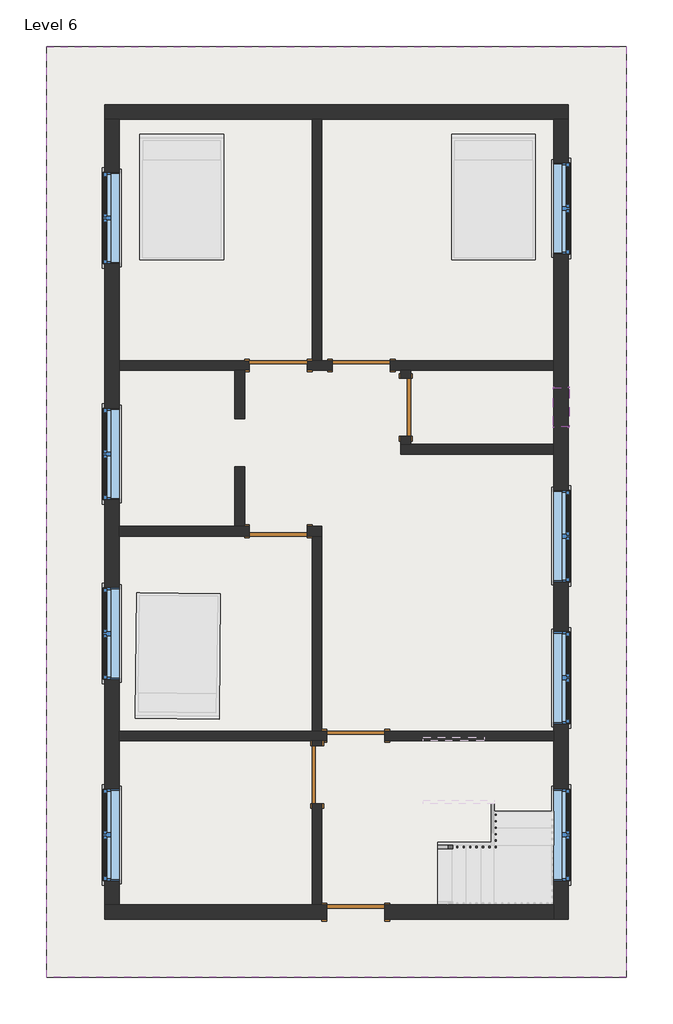
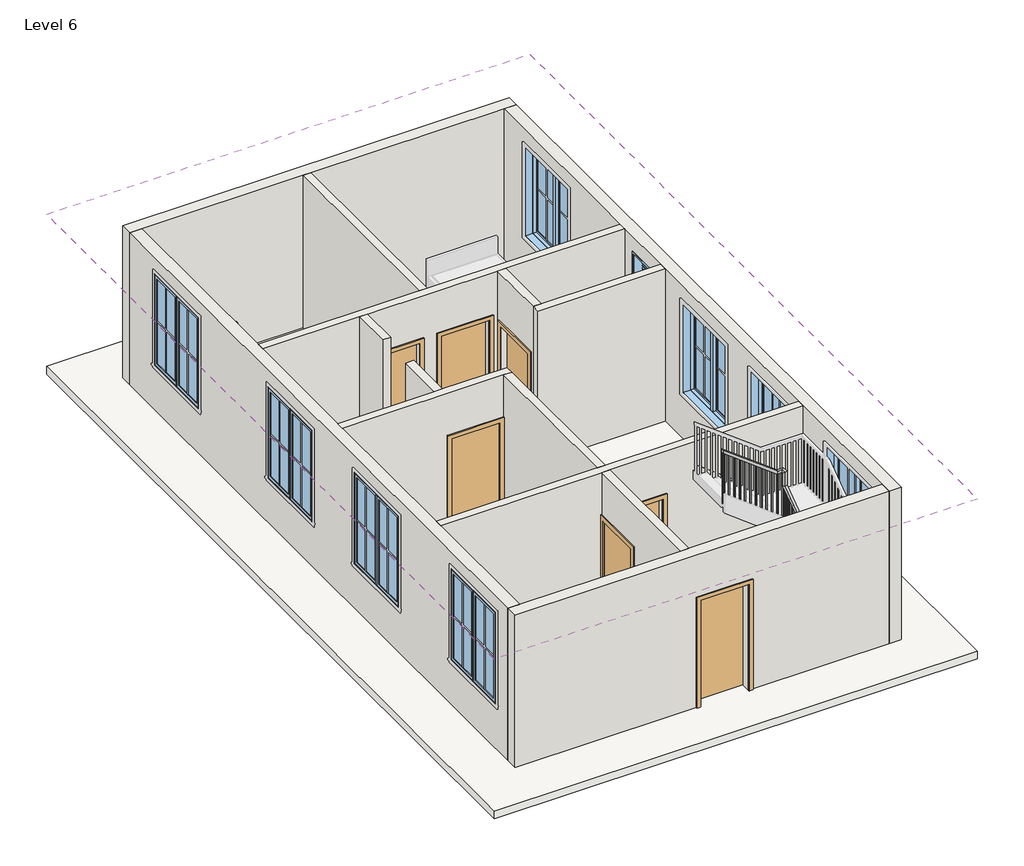
# One storey, part 1 of 2: 14 walls, 9 windows, 7 doors, 2 roofs, 1 railing.
"""IFC4 building model written with IfcOpenShell, lengths in millimetres."""

from ifc_helpers import new_model, si_unit, frame, origin, place, context, project, spatial, polyline, outline, extrude, faceted_brep, transform, mapped, element, save
from components import door_2b0b55a0, door_686f89d2, door_16372e1c, door_a90ba1ad, window_9ac97e1a, window_f2d8fef0

model = new_model("IFC4")

# Units and contexts
model_context = context("Model", 3, world=origin())
ifc_project = project(units=[si_unit("LENGTHUNIT", "METRE", prefix="MILLI")], contexts=[model_context])

# Site, building, storey
site = spatial("IfcSite", under=ifc_project)
building = spatial("IfcBuilding", under=site)
storey = spatial("IfcBuildingStorey", under=building, Name="Level 6", Elevation=12801.6)

# Doors
placement = place(None, origin())
door_shape = door_2b0b55a0(model_context)
element("IfcDoor", 1, ObjectType="Single-Flush : 36\" x 80\"", at=placement, inside=storey, context=model_context, shape_type="MappedRepresentation", body=[
    mapped(door_shape, transform((-163.235885, 1707.4649429, 12801.6), x_axis=(0.0, 1.0, 0.0), y_axis=(-1.0, 0.0, 0.0), z_axis=(0.0, 0.0, 1.0))),
])
door_2_shape = door_686f89d2(model_context)
element("IfcDoor", 2, ObjectType="Single-Flush : 36\" x 84\"", at=placement, inside=storey, context=model_context, shape_type="MappedRepresentation", body=[
    mapped(door_2_shape, transform((-861.735885, 2367.8649429, 12801.6), x_axis=(-1.0, 0.0, 0.0), y_axis=(0.0, -1.0, 0.0), z_axis=(0.0, 0.0, 1.0))),
])
element("IfcDoor", 3, ObjectType="Single-Flush : 36\" x 84\"", at=placement, inside=storey, context=model_context, shape_type="MappedRepresentation", body=[
    mapped(door_2_shape, transform((-2169.835885, -248.3350571, 12801.6), x_axis=(1.0, 0.0, 0.0), y_axis=(0.0, 1.0, 0.0), z_axis=(0.0, 0.0, 1.0))),
])
element("IfcDoor", 4, ObjectType="Single-Flush : 36\" x 84\"", at=placement, inside=storey, context=model_context, shape_type="MappedRepresentation", body=[
    mapped(door_2_shape, transform((-950.635885, -3474.1350571, 12801.6), x_axis=(-1.0, 0.0, 0.0), y_axis=(0.0, -1.0, 0.0), z_axis=(0.0, 0.0, 1.0))),
])
door_3_shape = door_16372e1c(model_context)
element("IfcDoor", 5, ObjectType="Single-Flush : 36\" x 84\"", at=placement, inside=storey, context=model_context, shape_type="MappedRepresentation", body=[
    mapped(door_3_shape, transform((-2169.835885, 2367.8649429, 12801.6), x_axis=(1.0, 0.0, 0.0), y_axis=(0.0, 1.0, 0.0), z_axis=(0.0, 0.0, 1.0))),
])
element("IfcDoor", 6, ObjectType="Single-Flush : 36\" x 84\"", at=placement, inside=storey, context=model_context, shape_type="MappedRepresentation", body=[
    mapped(door_3_shape, transform((-1560.235885, -4083.7350571, 12801.6), x_axis=(0.0, 1.0, 0.0), y_axis=(-1.0, 0.0, 0.0), z_axis=(0.0, 0.0, 1.0))),
])
door_4_shape = door_a90ba1ad(model_context)
element("IfcDoor", 7, ObjectType="Single-Flush : 36\" x 84\"", at=placement, inside=storey, context=model_context, shape_type="MappedRepresentation", body=[
    mapped(door_4_shape, transform((-950.635885, -6255.4350571, 12801.6), x_axis=(-1.0, 0.0, 0.0), y_axis=(0.0, -1.0, 0.0), z_axis=(0.0, 0.0, 1.0))),
])

# Railing
element("IfcRailing", 8, ObjectType="Handrail - Rectangular", at=placement, inside=storey, context=model_context, shape_type="SolidModel", body=[
    faceted_brep([(344.764115, -5201.3350571, 13885.3333333), (344.764115, -5201.3350571, 13821.4686436), (344.764115, -5252.1350571, 13821.4686436), (344.764115, -5252.1350571, 13885.3333333), (1157.564115, -5201.3350571, 14504.6095238), (1208.364115, -5201.3350571, 14479.449596), (1208.364115, -5252.1350571, 14479.449596), (1157.564115, -5252.1350571, 14504.6095238), (1157.564115, -5201.3350571, 14786.4285714), (1208.364115, -5201.3350571, 14735.6285714), (1208.364115, -5252.1350571, 14735.6285714), (1157.564115, -5252.1350571, 14786.4285714), (1233.764115, -5201.3350571, 14786.4285714), (1233.764115, -5201.3350571, 14735.6285714), (1284.564115, -5252.1350571, 14735.6285714), (1284.564115, -5252.1350571, 14786.4285714), (1233.764115, -5125.1350571, 14786.4285714), (1233.764115, -5108.8554323, 14735.6285714), (1284.564115, -5108.8554323, 14735.6285714), (1284.564115, -5125.1350571, 14786.4285714), (1233.764115, -4566.3350571, 15185.5714286), (1233.764115, -4515.5350571, 15159.4288395), (1284.564115, -4515.5350571, 15159.4288395), (1284.564115, -4566.3350571, 15185.5714286), (1233.764115, -4566.3350571, 15467.0606061), (1233.764115, -4515.5350571, 15416.2606061), (1284.564115, -4515.5350571, 15416.2606061), (1284.564115, -4566.3350571, 15467.0606061), (1233.764115, -4490.1350571, 15467.0606061), (1233.764115, -4490.1350571, 15416.2606061), (1284.564115, -4439.3350571, 15416.2606061), (1284.564115, -4439.3350571, 15467.0606061), (1157.564115, -4490.1350571, 15467.0606061), (1140.4943334, -4490.1350571, 15416.2606061), (1140.4943334, -4439.3350571, 15416.2606061), (1157.564115, -4439.3350571, 15467.0606061), (116.164115, -4490.1350571, 16256.0), (116.164115, -4439.3350571, 16256.0), (116.164115, -4439.3350571, 16192.2683472), (116.164115, -4490.1350571, 16192.2683472)], [[[0, 1, 2, 3]], [[1, 0, 4, 5]], [[2, 1, 5, 6]], [[3, 2, 6, 7]], [[0, 3, 7, 4]], [[5, 4, 8, 9]], [[6, 5, 9, 10]], [[7, 6, 10, 11]], [[4, 7, 11, 8]], [[9, 8, 12, 13]], [[10, 9, 13, 14]], [[11, 10, 14, 15]], [[8, 11, 15, 12]], [[13, 12, 16, 17]], [[14, 13, 17, 18]], [[15, 14, 18, 19]], [[12, 15, 19, 16]], [[17, 16, 20, 21]], [[18, 17, 21, 22]], [[19, 18, 22, 23]], [[16, 19, 23, 20]], [[21, 20, 24, 25]], [[22, 21, 25, 26]], [[23, 22, 26, 27]], [[20, 23, 27, 24]], [[25, 24, 28, 29]], [[26, 25, 29, 30]], [[27, 26, 30, 31]], [[24, 27, 31, 28]], [[29, 28, 32, 33]], [[30, 29, 33, 34]], [[31, 30, 34, 35]], [[28, 31, 35, 32]], [[36, 37, 38, 39]], [[33, 32, 36, 39]], [[34, 33, 39, 38]], [[35, 34, 38, 37]], [[32, 35, 37, 36]]]),
    extrude(outline(polyline([(16180.2418321, 132.039115), (15172.2666667, 132.039115), (15172.2666667, 151.089115), (16165.8100139, 151.089115), (16180.2418321, 132.039115)])), frame((0.0, -4474.2600571, 0.0), z_axis=(0.0, 1.0, 0.0), x_axis=(0.0, 0.0, 1.0)), (0.0, 0.0, 1.0), 19.05),
    extrude(outline(polyline([(16103.2721351, 233.639115), (15172.2666667, 233.639115), (15172.2666667, 252.689115), (16088.8403169, 252.689115), (16103.2721351, 233.639115)])), frame((0.0, -4474.2600571, 0.0), z_axis=(0.0, 1.0, 0.0), x_axis=(0.0, 0.0, 1.0)), (0.0, 0.0, 1.0), 19.05),
    extrude(outline(polyline([(16026.3024382, 335.239115), (15172.2666667, 335.239115), (15172.2666667, 354.289115), (16011.87062, 354.289115), (16026.3024382, 335.239115)])), frame((0.0, -4474.2600571, 0.0), z_axis=(0.0, 1.0, 0.0), x_axis=(0.0, 0.0, 1.0)), (0.0, 0.0, 1.0), 19.05),
    extrude(outline(polyline([(15949.3327412, 436.839115), (15002.9333333, 436.839115), (15002.9333333, 455.889115), (15934.900923, 455.889115), (15949.3327412, 436.839115)])), frame((0.0, -4474.2600571, 0.0), z_axis=(0.0, 1.0, 0.0), x_axis=(0.0, 0.0, 1.0)), (0.0, 0.0, 1.0), 19.05),
    extrude(outline(polyline([(15872.3630442, 538.439115), (15002.9333333, 538.439115), (15002.9333333, 557.489115), (15857.931226, 557.489115), (15872.3630442, 538.439115)])), frame((0.0, -4474.2600571, 0.0), z_axis=(0.0, 1.0, 0.0), x_axis=(0.0, 0.0, 1.0)), (0.0, 0.0, 1.0), 19.05),
    extrude(outline(polyline([(15795.3933472, 640.039115), (14833.6, 640.039115), (14833.6, 659.089115), (15780.9615291, 659.089115), (15795.3933472, 640.039115)])), frame((0.0, -4474.2600571, 0.0), z_axis=(0.0, 1.0, 0.0), x_axis=(0.0, 0.0, 1.0)), (0.0, 0.0, 1.0), 19.05),
    extrude(outline(polyline([(15718.4236503, 741.639115), (14833.6, 741.639115), (14833.6, 760.689115), (15703.9918321, 760.689115), (15718.4236503, 741.639115)])), frame((0.0, -4474.2600571, 0.0), z_axis=(0.0, 1.0, 0.0), x_axis=(0.0, 0.0, 1.0)), (0.0, 0.0, 1.0), 19.05),
    extrude(outline(polyline([(15641.4539533, 843.239115), (14664.2666667, 843.239115), (14664.2666667, 862.289115), (15627.0221351, 862.289115), (15641.4539533, 843.239115)])), frame((0.0, -4474.2600571, 0.0), z_axis=(0.0, 1.0, 0.0), x_axis=(0.0, 0.0, 1.0)), (0.0, 0.0, 1.0), 19.05),
    extrude(outline(polyline([(15564.4842563, 944.839115), (14664.2666667, 944.839115), (14664.2666667, 963.889115), (15550.0524382, 963.889115), (15564.4842563, 944.839115)])), frame((0.0, -4474.2600571, 0.0), z_axis=(0.0, 1.0, 0.0), x_axis=(0.0, 0.0, 1.0)), (0.0, 0.0, 1.0), 19.05),
    extrude(outline(polyline([(15487.5145594, 1046.439115), (14494.9333333, 1046.439115), (14494.9333333, 1065.489115), (15473.0827412, 1065.489115), (15487.5145594, 1046.439115)])), frame((0.0, -4474.2600571, 0.0), z_axis=(0.0, 1.0, 0.0), x_axis=(0.0, 0.0, 1.0)), (0.0, 0.0, 1.0), 19.05),
    extrude(outline(polyline([(15410.5448624, 1148.039115), (14494.9333333, 1148.039115), (14494.9333333, 1167.089115), (15396.1130442, 1167.089115), (15410.5448624, 1148.039115)])), frame((0.0, -4474.2600571, 0.0), z_axis=(0.0, 1.0, 0.0), x_axis=(0.0, 0.0, 1.0)), (0.0, 0.0, 1.0), 19.05),
    extrude(outline(polyline([(1249.639115, -4525.0600571), (1249.639115, -4506.0100571), (1268.689115, -4506.0100571), (1268.689115, -4525.0600571), (1249.639115, -4525.0600571)])), frame((0.0, 0.0, 14156.2666667), z_axis=(0.0, 0.0, 1.0), x_axis=(1.0, 0.0, 0.0)), (0.0, 0.0, 1.0), 1259.9939394),
    extrude(outline(polyline([(-4607.6100571, 15093.6609823), (-4607.6100571, 14156.2666667), (-4626.6600571, 14156.2666667), (-4626.6600571, 15080.0538395), (-4607.6100571, 15093.6609823)])), frame((1249.639115, 0.0, 0.0), z_axis=(1.0, 0.0, 0.0), x_axis=(0.0, 1.0, 0.0)), (0.0, 0.0, 1.0), 19.05),
    extrude(outline(polyline([(-4709.2100571, 15021.0895538), (-4709.2100571, 13986.9333333), (-4728.2600571, 13986.9333333), (-4728.2600571, 15007.4824109), (-4709.2100571, 15021.0895538)])), frame((1249.639115, 0.0, 0.0), z_axis=(1.0, 0.0, 0.0), x_axis=(0.0, 1.0, 0.0)), (0.0, 0.0, 1.0), 19.05),
    extrude(outline(polyline([(-4810.8100571, 14948.5181252), (-4810.8100571, 13986.9333333), (-4829.8600571, 13986.9333333), (-4829.8600571, 14934.9109823), (-4810.8100571, 14948.5181252)])), frame((1249.639115, 0.0, 0.0), z_axis=(1.0, 0.0, 0.0), x_axis=(0.0, 1.0, 0.0)), (0.0, 0.0, 1.0), 19.05),
    extrude(outline(polyline([(-4912.4100571, 14875.9466966), (-4912.4100571, 13986.9333333), (-4931.4600571, 13986.9333333), (-4931.4600571, 14862.3395538), (-4912.4100571, 14875.9466966)])), frame((1249.639115, 0.0, 0.0), z_axis=(1.0, 0.0, 0.0), x_axis=(0.0, 1.0, 0.0)), (0.0, 0.0, 1.0), 19.05),
    extrude(outline(polyline([(-5014.0100571, 14803.3752681), (-5014.0100571, 13817.6), (-5033.0600571, 13817.6), (-5033.0600571, 14789.7681252), (-5014.0100571, 14803.3752681)])), frame((1249.639115, 0.0, 0.0), z_axis=(1.0, 0.0, 0.0), x_axis=(0.0, 1.0, 0.0)), (0.0, 0.0, 1.0), 19.05),
    extrude(outline(polyline([(-5115.6100571, 14730.8038395), (-5115.6100571, 13817.6), (-5134.6600571, 13817.6), (-5134.6600571, 14717.1966966), (-5115.6100571, 14730.8038395)])), frame((1249.639115, 0.0, 0.0), z_axis=(1.0, 0.0, 0.0), x_axis=(0.0, 1.0, 0.0)), (0.0, 0.0, 1.0), 19.05),
    extrude(outline(polyline([(14433.4876912, 1148.039115), (13478.9333333, 1148.039115), (13478.9333333, 1167.089115), (14448.0019769, 1167.089115), (14433.4876912, 1148.039115)])), frame((0.0, -5236.2600571, 0.0), z_axis=(0.0, 1.0, 0.0), x_axis=(0.0, 0.0, 1.0)), (0.0, 0.0, 1.0), 19.05),
    extrude(outline(polyline([(14356.0781674, 1046.439115), (13478.9333333, 1046.439115), (13478.9333333, 1065.489115), (14370.5924531, 1065.489115), (14356.0781674, 1046.439115)])), frame((0.0, -5236.2600571, 0.0), z_axis=(0.0, 1.0, 0.0), x_axis=(0.0, 0.0, 1.0)), (0.0, 0.0, 1.0), 19.05),
    extrude(outline(polyline([(14278.6686436, 944.839115), (13309.6, 944.839115), (13309.6, 963.889115), (14293.1829293, 963.889115), (14278.6686436, 944.839115)])), frame((0.0, -5236.2600571, 0.0), z_axis=(0.0, 1.0, 0.0), x_axis=(0.0, 0.0, 1.0)), (0.0, 0.0, 1.0), 19.05),
    extrude(outline(polyline([(14201.2591198, 843.239115), (13309.6, 843.239115), (13309.6, 862.289115), (14215.7734055, 862.289115), (14201.2591198, 843.239115)])), frame((0.0, -5236.2600571, 0.0), z_axis=(0.0, 1.0, 0.0), x_axis=(0.0, 0.0, 1.0)), (0.0, 0.0, 1.0), 19.05),
    extrude(outline(polyline([(14123.849596, 741.639115), (13140.2666667, 741.639115), (13140.2666667, 760.689115), (14138.3638817, 760.689115), (14123.849596, 741.639115)])), frame((0.0, -5236.2600571, 0.0), z_axis=(0.0, 1.0, 0.0), x_axis=(0.0, 0.0, 1.0)), (0.0, 0.0, 1.0), 19.05),
    extrude(outline(polyline([(14046.4400722, 640.039115), (13140.2666667, 640.039115), (13140.2666667, 659.089115), (14060.9543579, 659.089115), (14046.4400722, 640.039115)])), frame((0.0, -5236.2600571, 0.0), z_axis=(0.0, 1.0, 0.0), x_axis=(0.0, 0.0, 1.0)), (0.0, 0.0, 1.0), 19.05),
    extrude(outline(polyline([(13969.0305484, 538.439115), (12970.9333333, 538.439115), (12970.9333333, 557.489115), (13983.5448341, 557.489115), (13969.0305484, 538.439115)])), frame((0.0, -5236.2600571, 0.0), z_axis=(0.0, 1.0, 0.0), x_axis=(0.0, 0.0, 1.0)), (0.0, 0.0, 1.0), 19.05),
    extrude(outline(polyline([(13891.6210246, 436.839115), (12970.9333333, 436.839115), (12970.9333333, 455.889115), (13906.1353103, 455.889115), (13891.6210246, 436.839115)])), frame((0.0, -5236.2600571, 0.0), z_axis=(0.0, 1.0, 0.0), x_axis=(0.0, 0.0, 1.0)), (0.0, 0.0, 1.0), 19.05),
    extrude(outline(polyline([(1249.639115, -4474.2600571), (1249.639115, -4455.2100571), (1268.689115, -4455.2100571), (1268.689115, -4474.2600571), (1249.639115, -4474.2600571)])), frame((0.0, 0.0, 14325.6), z_axis=(0.0, 0.0, 1.0), x_axis=(1.0, 0.0, 0.0)), (0.0, 0.0, 1.0), 1090.6606061),
    extrude(outline(polyline([(1249.639115, -5217.2100571), (1268.689115, -5217.2100571), (1268.689115, -5236.2600571), (1249.639115, -5236.2600571), (1249.639115, -5217.2100571)])), frame((0.0, 0.0, 13648.2666667), z_axis=(0.0, 0.0, 1.0), x_axis=(1.0, 0.0, 0.0)), (0.0, 0.0, 1.0), 1087.3619048),
    extrude(outline(polyline([(16192.2683472, 116.164115), (15172.2666667, 116.164115), (15172.2666667, 135.214115), (16177.8365291, 135.214115), (16192.2683472, 116.164115)])), frame((0.0, -4474.2600571, 0.0), z_axis=(0.0, 1.0, 0.0), x_axis=(0.0, 0.0, 1.0)), (0.0, 0.0, 1.0), 19.05),
    extrude(outline(polyline([(13821.4686436, 344.764115), (12970.9333333, 344.764115), (12970.9333333, 363.814115), (13835.9829293, 363.814115), (13821.4686436, 344.764115)])), frame((0.0, -5236.2600571, 0.0), z_axis=(0.0, 1.0, 0.0), x_axis=(0.0, 0.0, 1.0)), (0.0, 0.0, 1.0), 19.05),
])

# Roofs
element("IfcRoof", 9, ObjectType="ROOF 6\"", at=placement, inside=storey, context=model_context, shape_type="SweptSolid", body=[
    extrude(outline(polyline([(-5827.435885, 7397.0649429), (3316.564115, 7397.0649429), (3316.564115, -7284.1350571), (-5827.435885, -7284.1350571), (-5827.435885, 7397.0649429)])), frame((0.0, 0.0, 12649.2), z_axis=(0.0, 0.0, 1.0), x_axis=(1.0, 0.0, 0.0)), (0.0, 0.0, 1.0), 152.4),
])
element("IfcRoof", 10, ObjectType="ROOF 6\"", at=placement, inside=storey, context=model_context, shape_type="SweptSolid", body=[
    extrude(outline(polyline([(-5827.435885, 7397.0649429), (3316.564115, 7397.0649429), (3316.564115, -7284.1350571), (-5827.435885, -7284.1350571), (-5827.435885, 7397.0649429)])), frame((0.0, 0.0, 15849.6), z_axis=(0.0, 0.0, 1.0), x_axis=(1.0, 0.0, 0.0)), (0.0, 0.0, 1.0), 152.4),
])

# Walls
element("IfcWall", 11, ObjectType="WALL 6\"", at=placement, inside=storey, context=model_context, shape_type="SweptSolid", body=[
    extrude(outline(polyline([(-1636.435885, 2444.0649429), (-1636.435885, 6254.0649429), (-1484.035885, 6254.0649429), (-1484.035885, 2444.0649429), (-1636.435885, 2444.0649429)])), frame((0.0, 0.0, 12801.6), z_axis=(0.0, 0.0, 1.0), x_axis=(1.0, 0.0, 0.0)), (0.0, 0.0, 1.0), 3048.0),
])
element("IfcWall", 12, ObjectType="WALL 6\"", at=placement, inside=storey, context=model_context, shape_type="Brep", body=[
    faceted_brep([(-1318.935885, 2444.0649429, 12801.6), (-1484.035885, 2444.0649429, 12801.6), (-1636.435885, 2444.0649429, 12801.6), (-1712.635885, 2444.0649429, 12801.6), (-1712.635885, 2444.0649429, 14935.2), (-2627.035885, 2444.0649429, 14935.2), (-2627.035885, 2444.0649429, 12801.6), (-4684.435885, 2444.0649429, 12801.6), (-4684.435885, 2444.0649429, 15849.6), (-1636.435885, 2444.0649429, 15849.6), (-1484.035885, 2444.0649429, 15849.6), (2173.564115, 2444.0649429, 15849.6), (2173.564115, 2444.0649429, 12801.6), (-404.535885, 2444.0649429, 12801.6), (-404.535885, 2444.0649429, 14935.2), (-1318.935885, 2444.0649429, 14935.2), (-1712.635885, 2291.6649429, 14935.2), (-1712.635885, 2291.6649429, 12801.6), (-1318.935885, 2291.6649429, 12801.6), (-1318.935885, 2291.6649429, 14935.2), (-404.535885, 2291.6649429, 14935.2), (-404.535885, 2291.6649429, 12801.6), (-239.435885, 2291.6649429, 12801.6), (-87.035885, 2291.6649429, 12801.6), (2173.564115, 2291.6649429, 12801.6), (2173.564115, 2291.6649429, 15849.6), (-87.035885, 2291.6649429, 15849.6), (-239.435885, 2291.6649429, 15849.6), (-2703.235885, 2291.6649429, 15849.6), (-2855.635885, 2291.6649429, 15849.6), (-4684.435885, 2291.6649429, 15849.6), (-4684.435885, 2291.6649429, 12801.6), (-2855.635885, 2291.6649429, 12801.6), (-2703.235885, 2291.6649429, 12801.6), (-2627.035885, 2291.6649429, 12801.6), (-2627.035885, 2291.6649429, 14935.2)], [[[0, 1, 2, 3, 4, 5, 6, 7, 8, 9, 10, 11, 12, 13, 14, 15]], [[16, 17, 18, 19, 20, 21, 22, 23, 24, 25, 26, 27, 28, 29, 30, 31, 32, 33, 34, 35]], [[13, 12, 24, 23, 22, 21]], [[18, 17, 3, 2, 1, 0]], [[34, 33, 32, 31, 7, 6]], [[12, 11, 25, 24]], [[8, 7, 31, 30]], [[19, 18, 0, 15]], [[20, 19, 15, 14]], [[21, 20, 14, 13]], [[4, 3, 17, 16]], [[5, 4, 16, 35]], [[6, 5, 35, 34]], [[11, 10, 9, 8, 30, 29, 28, 27, 26, 25]]]),
])
element("IfcWall", 13, ObjectType="WALL 6\"", at=placement, inside=storey, context=model_context, shape_type="SweptSolid", body=[
    extrude(outline(polyline([(-2855.635885, 1529.6649429), (-2855.635885, 2291.6649429), (-2703.235885, 2291.6649429), (-2703.235885, 1529.6649429), (-2855.635885, 1529.6649429)])), frame((0.0, 0.0, 12801.6), z_axis=(0.0, 0.0, 1.0), x_axis=(1.0, 0.0, 0.0)), (0.0, 0.0, 1.0), 3048.0),
])
element("IfcWall", 14, ObjectType="WALL 6\"", at=placement, inside=storey, context=model_context, shape_type="Brep", body=[
    faceted_brep([(-1712.635885, -324.5350571, 14935.2), (-1712.635885, -324.5350571, 12801.6), (-1636.435885, -324.5350571, 12801.6), (-1484.035885, -324.5350571, 12801.6), (-1484.035885, -324.5350571, 15849.6), (-1636.435885, -324.5350571, 15849.6), (-4684.435885, -324.5350571, 15849.6), (-4684.435885, -324.5350571, 12801.6), (-2627.035885, -324.5350571, 12801.6), (-2627.035885, -324.5350571, 14935.2), (-1484.035885, -172.1350571, 12801.6), (-1712.635885, -172.1350571, 12801.6), (-1712.635885, -172.1350571, 14935.2), (-2627.035885, -172.1350571, 14935.2), (-2627.035885, -172.1350571, 12801.6), (-2703.235885, -172.1350571, 12801.6), (-2855.635885, -172.1350571, 12801.6), (-4684.435885, -172.1350571, 12801.6), (-4684.435885, -172.1350571, 15849.6), (-2855.635885, -172.1350571, 15849.6), (-2703.235885, -172.1350571, 15849.6), (-1484.035885, -172.1350571, 15849.6)], [[[0, 1, 2, 3, 4, 5, 6, 7, 8, 9]], [[10, 11, 12, 13, 14, 15, 16, 17, 18, 19, 20, 21]], [[8, 7, 17, 16, 15, 14]], [[3, 2, 1, 11, 10]], [[7, 6, 18, 17]], [[4, 3, 10, 21]], [[12, 11, 1, 0]], [[13, 12, 0, 9]], [[14, 13, 9, 8]], [[6, 5, 4, 21, 20, 19, 18]]]),
])
element("IfcWall", 15, ObjectType="WALL 6\"", at=placement, inside=storey, context=model_context, shape_type="SweptSolid", body=[
    extrude(outline(polyline([(-1636.435885, -3397.9350571), (-1636.435885, -324.5350571), (-1484.035885, -324.5350571), (-1484.035885, -3397.9350571), (-1636.435885, -3397.9350571)])), frame((0.0, 0.0, 12801.6), z_axis=(0.0, 0.0, 1.0), x_axis=(1.0, 0.0, 0.0)), (0.0, 0.0, 1.0), 3048.0),
])
element("IfcWall", 16, ObjectType="WALL 6\"", at=placement, inside=storey, context=model_context, shape_type="Brep", body=[
    faceted_brep([(-4684.435885, -3550.3350571, 12801.6), (-1636.435885, -3550.3350571, 12801.6), (-1484.035885, -3550.3350571, 12801.6), (-1407.835885, -3550.3350571, 12801.6), (-1407.835885, -3550.3350571, 14935.2), (-493.435885, -3550.3350571, 14935.2), (-493.435885, -3550.3350571, 12801.6), (2173.564115, -3550.3350571, 12801.6), (2173.564115, -3550.3350571, 15849.6), (-1484.035885, -3550.3350571, 15849.6), (-1636.435885, -3550.3350571, 15849.6), (-4684.435885, -3550.3350571, 15849.6), (-1407.835885, -3397.9350571, 14935.2), (-1407.835885, -3397.9350571, 12801.6), (-1484.035885, -3397.9350571, 12801.6), (-1636.435885, -3397.9350571, 12801.6), (-4684.435885, -3397.9350571, 12801.6), (-4684.435885, -3397.9350571, 15849.6), (-1636.435885, -3397.9350571, 15849.6), (-1484.035885, -3397.9350571, 15849.6), (2173.564115, -3397.9350571, 15849.6), (2173.564115, -3397.9350571, 12801.6), (-493.435885, -3397.9350571, 12801.6), (-493.435885, -3397.9350571, 14935.2)], [[[0, 1, 2, 3, 4, 5, 6, 7, 8, 9, 10, 11]], [[12, 13, 14, 15, 16, 17, 18, 19, 20, 21, 22, 23]], [[22, 21, 7, 6]], [[16, 15, 14, 13, 3, 2, 1, 0]], [[8, 7, 21, 20]], [[0, 11, 17, 16]], [[4, 3, 13, 12]], [[5, 4, 12, 23]], [[6, 5, 23, 22]], [[11, 10, 9, 8, 20, 19, 18, 17]]]),
])
element("IfcWall", 17, ObjectType="WALL 6\"", at=placement, inside=storey, context=model_context, shape_type="SweptSolid", body=[
    extrude(outline(polyline([(-3550.3350571, 12801.6), (-3626.5350571, 12801.6), (-3626.5350571, 14935.2), (-4540.9350571, 14935.2), (-4540.9350571, 12801.6), (-6141.1350571, 12801.6), (-6141.1350571, 15849.6), (-3550.3350571, 15849.6), (-3550.3350571, 12801.6)])), frame((-1636.435885, 0.0, 0.0), z_axis=(1.0, 0.0, 0.0), x_axis=(0.0, 1.0, 0.0)), (0.0, 0.0, 1.0), 152.4),
])
element("IfcWall", 18, ObjectType="WALL 6\"", at=placement, inside=storey, context=model_context, shape_type="Brep", body=[
    faceted_brep([(2173.564115, 1123.2649429, 12801.6), (-87.035885, 1123.2649429, 12801.6), (-239.435885, 1123.2649429, 12801.6), (-239.435885, 1123.2649429, 15849.6), (-87.035885, 1123.2649429, 15849.6), (2173.564115, 1123.2649429, 15849.6), (2173.564115, 970.8649429, 12801.6), (2173.564115, 970.8649429, 15849.6), (-239.435885, 970.8649429, 15849.6), (-239.435885, 970.8649429, 12801.6)], [[[0, 1, 2, 3, 4, 5]], [[6, 7, 8, 9]], [[2, 1, 0, 6, 9]], [[0, 5, 7, 6]], [[3, 2, 9, 8]], [[5, 4, 3, 8, 7]]]),
])
element("IfcWall", 19, ObjectType="WALL 6\"", at=placement, inside=storey, context=model_context, shape_type="SweptSolid", body=[
    extrude(outline(polyline([(2291.6649429, 12801.6), (2164.6649429, 12801.6), (2164.6649429, 14833.6), (1250.2649429, 14833.6), (1250.2649429, 12801.6), (1123.2649429, 12801.6), (1123.2649429, 15849.6), (2291.6649429, 15849.6), (2291.6649429, 12801.6)])), frame((-239.435885, 0.0, 0.0), z_axis=(1.0, 0.0, 0.0), x_axis=(0.0, 1.0, 0.0)), (0.0, 0.0, 1.0), 152.4),
])
element("IfcWall", 20, ObjectType="WALL 6\"", at=placement, inside=storey, context=model_context, shape_type="SweptSolid", body=[
    extrude(outline(polyline([(-2855.635885, -172.1350571), (-2855.635885, 767.6649429), (-2703.235885, 767.6649429), (-2703.235885, -172.1350571), (-2855.635885, -172.1350571)])), frame((0.0, 0.0, 12801.6), z_axis=(0.0, 0.0, 1.0), x_axis=(1.0, 0.0, 0.0)), (0.0, 0.0, 1.0), 3048.0),
])
element("IfcWall", 21, ObjectType="WALL 9\"", at=placement, inside=storey, context=model_context, shape_type="Brep", body=[
    faceted_brep([(-4913.035885, 6254.0649429, 12801.6), (-4684.435885, 6254.0649429, 12801.6), (-1636.435885, 6254.0649429, 12801.6), (-1484.035885, 6254.0649429, 12801.6), (2173.564115, 6254.0649429, 12801.6), (2402.164115, 6254.0649429, 12801.6), (2402.164115, 6254.0649429, 15849.6), (2173.564115, 6254.0649429, 15849.6), (-1484.035885, 6254.0649429, 15849.6), (-1636.435885, 6254.0649429, 15849.6), (-4684.435885, 6254.0649429, 15849.6), (-4913.035885, 6254.0649429, 15849.6), (-4913.035885, 6482.6649429, 12801.6), (-4913.035885, 6482.6649429, 15849.6), (2402.164115, 6482.6649429, 15849.6), (2402.164115, 6482.6649429, 12801.6)], [[[0, 1, 2, 3, 4, 5, 6, 7, 8, 9, 10, 11]], [[12, 13, 14, 15]], [[5, 4, 3, 2, 1, 0, 12, 15]], [[6, 5, 15, 14]], [[0, 11, 13, 12]], [[11, 10, 9, 8, 7, 6, 14, 13]]]),
])
element("IfcWall", 22, ObjectType="WALL 9\"", at=placement, inside=storey, context=model_context, shape_type="Brep", body=[
    faceted_brep([(2173.564115, 6254.0649429, 12801.6), (2173.564115, 2444.0649429, 12801.6), (2173.564115, 2291.6649429, 12801.6), (2173.564115, 1123.2649429, 12801.6), (2173.564115, 970.8649429, 12801.6), (2173.564115, -3397.9350571, 12801.6), (2173.564115, -3550.3350571, 12801.6), (2173.564115, -6141.1350571, 12801.6), (2173.564115, -6369.7350571, 12801.6), (2173.564115, -6369.7350571, 15849.6), (2173.564115, -6141.1350571, 15849.6), (2173.564115, -3550.3350571, 15849.6), (2173.564115, -3397.9350571, 15849.6), (2173.564115, 970.8649429, 15849.6), (2173.564115, 1123.2649429, 15849.6), (2173.564115, 2291.6649429, 15849.6), (2173.564115, 2444.0649429, 15849.6), (2173.564115, 6254.0649429, 15849.6), (2173.564115, -5760.1350571, 15544.8), (2173.564115, -5760.1350571, 13716.0), (2173.564115, -4312.3350571, 13716.0), (2173.564115, -4312.3350571, 15544.8), (2173.564115, -3283.6350571, 15544.8), (2173.564115, -3283.6350571, 13716.0), (2173.564115, -1835.8350571, 13716.0), (2173.564115, -1835.8350571, 15544.8), (2173.564115, -1048.4350571, 15544.8), (2173.564115, -1048.4350571, 13716.0), (2173.564115, 399.3649429, 13716.0), (2173.564115, 399.3649429, 15544.8), (2173.564115, 4120.4649429, 15544.8), (2173.564115, 4120.4649429, 13716.0), (2173.564115, 5568.2649429, 13716.0), (2173.564115, 5568.2649429, 15544.8), (2173.564115, 2012.2649429, 15544.8), (2173.564115, 1402.6649429, 15544.8), (2173.564115, 1402.6649429, 14935.2), (2173.564115, 2012.2649429, 14935.2), (2402.164115, 6254.0649429, 12801.6), (2402.164115, 6254.0649429, 15849.6), (2402.164115, -6369.7350571, 15849.6), (2402.164115, -6369.7350571, 12801.6), (2402.164115, -5760.1350571, 15544.8), (2402.164115, -4312.3350571, 15544.8), (2402.164115, -4312.3350571, 13716.0), (2402.164115, -5760.1350571, 13716.0), (2402.164115, -3283.6350571, 15544.8), (2402.164115, -1835.8350571, 15544.8), (2402.164115, -1835.8350571, 13716.0), (2402.164115, -3283.6350571, 13716.0), (2402.164115, -1048.4350571, 15544.8), (2402.164115, 399.3649429, 15544.8), (2402.164115, 399.3649429, 13716.0), (2402.164115, -1048.4350571, 13716.0), (2402.164115, 4120.4649429, 15544.8), (2402.164115, 5568.2649429, 15544.8), (2402.164115, 5568.2649429, 13716.0), (2402.164115, 4120.4649429, 13716.0), (2402.164115, 2012.2649429, 15544.8), (2402.164115, 2012.2649429, 14935.2), (2402.164115, 1402.6649429, 14935.2), (2402.164115, 1402.6649429, 15544.8)], [[[0, 1, 2, 3, 4, 5, 6, 7, 8, 9, 10, 11, 12, 13, 14, 15, 16, 17], [18, 19, 20, 21], [22, 23, 24, 25], [26, 27, 28, 29], [30, 31, 32, 33], [34, 35, 36, 37]], [[38, 39, 40, 41], [42, 43, 44, 45], [46, 47, 48, 49], [50, 51, 52, 53], [54, 55, 56, 57], [58, 59, 60, 61]], [[8, 7, 6, 5, 4, 3, 2, 1, 0, 38, 41]], [[0, 17, 39, 38]], [[9, 8, 41, 40]], [[19, 18, 42, 45]], [[20, 19, 45, 44]], [[21, 20, 44, 43]], [[18, 21, 43, 42]], [[23, 22, 46, 49]], [[24, 23, 49, 48]], [[25, 24, 48, 47]], [[22, 25, 47, 46]], [[27, 26, 50, 53]], [[28, 27, 53, 52]], [[29, 28, 52, 51]], [[26, 29, 51, 50]], [[31, 30, 54, 57]], [[32, 31, 57, 56]], [[33, 32, 56, 55]], [[30, 33, 55, 54]], [[59, 58, 34, 37]], [[60, 59, 37, 36]], [[61, 60, 36, 35]], [[58, 61, 35, 34]], [[17, 16, 15, 14, 13, 12, 11, 10, 9, 40, 39]]]),
])
element("IfcWall", 23, ObjectType="WALL 9\"", at=placement, inside=storey, context=model_context, shape_type="Brep", body=[
    faceted_brep([(-1407.835885, -6141.1350571, 14935.2), (-1407.835885, -6141.1350571, 12801.6), (-1484.035885, -6141.1350571, 12801.6), (-1636.435885, -6141.1350571, 12801.6), (-4684.435885, -6141.1350571, 12801.6), (-4913.035885, -6141.1350571, 12801.6), (-4913.035885, -6141.1350571, 15849.6), (-4684.435885, -6141.1350571, 15849.6), (-1636.435885, -6141.1350571, 15849.6), (-1484.035885, -6141.1350571, 15849.6), (2173.564115, -6141.1350571, 15849.6), (2173.564115, -6141.1350571, 12801.6), (-493.435885, -6141.1350571, 12801.6), (-493.435885, -6141.1350571, 14935.2), (-4913.035885, -6369.7350571, 12801.6), (-1407.835885, -6369.7350571, 12801.6), (-1407.835885, -6369.7350571, 14935.2), (-493.435885, -6369.7350571, 14935.2), (-493.435885, -6369.7350571, 12801.6), (2173.564115, -6369.7350571, 12801.6), (2173.564115, -6369.7350571, 15849.6), (-4913.035885, -6369.7350571, 15849.6)], [[[0, 1, 2, 3, 4, 5, 6, 7, 8, 9, 10, 11, 12, 13]], [[14, 15, 16, 17, 18, 19, 20, 21]], [[12, 11, 19, 18]], [[5, 4, 3, 2, 1, 15, 14]], [[11, 10, 20, 19]], [[6, 5, 14, 21]], [[16, 15, 1, 0]], [[17, 16, 0, 13]], [[18, 17, 13, 12]], [[10, 9, 8, 7, 6, 21, 20]]]),
])
element("IfcWall", 24, ObjectType="WALL 9\"", at=placement, inside=storey, context=model_context, shape_type="Brep", body=[
    faceted_brep([(-4684.435885, -6141.1350571, 12801.6), (-4684.435885, -3550.3350571, 12801.6), (-4684.435885, -3397.9350571, 12801.6), (-4684.435885, -324.5350571, 12801.6), (-4684.435885, -172.1350571, 12801.6), (-4684.435885, 2291.6649429, 12801.6), (-4684.435885, 2444.0649429, 12801.6), (-4684.435885, 6254.0649429, 12801.6), (-4684.435885, 6254.0649429, 15849.6), (-4684.435885, 2444.0649429, 15849.6), (-4684.435885, 2291.6649429, 15849.6), (-4684.435885, -172.1350571, 15849.6), (-4684.435885, -324.5350571, 15849.6), (-4684.435885, -3397.9350571, 15849.6), (-4684.435885, -3550.3350571, 15849.6), (-4684.435885, -6141.1350571, 15849.6), (-4684.435885, -4312.3350571, 15544.8), (-4684.435885, -4312.3350571, 13716.0), (-4684.435885, -5760.1350571, 13716.0), (-4684.435885, -5760.1350571, 15544.8), (-4684.435885, -1137.3350571, 15544.8), (-4684.435885, -1137.3350571, 13716.0), (-4684.435885, -2585.1350571, 13716.0), (-4684.435885, -2585.1350571, 15544.8), (-4684.435885, 1694.7649429, 15544.8), (-4684.435885, 1694.7649429, 13716.0), (-4684.435885, 246.9649429, 13716.0), (-4684.435885, 246.9649429, 15544.8), (-4684.435885, 5415.8649429, 15544.8), (-4684.435885, 5415.8649429, 13716.0), (-4684.435885, 3968.0649429, 13716.0), (-4684.435885, 3968.0649429, 15544.8), (-4913.035885, -6141.1350571, 12801.6), (-4913.035885, -6141.1350571, 15849.6), (-4913.035885, 6254.0649429, 15849.6), (-4913.035885, 6254.0649429, 12801.6), (-4913.035885, -4312.3350571, 15544.8), (-4913.035885, -5760.1350571, 15544.8), (-4913.035885, -5760.1350571, 13716.0), (-4913.035885, -4312.3350571, 13716.0), (-4913.035885, -1137.3350571, 15544.8), (-4913.035885, -2585.1350571, 15544.8), (-4913.035885, -2585.1350571, 13716.0), (-4913.035885, -1137.3350571, 13716.0), (-4913.035885, 1694.7649429, 15544.8), (-4913.035885, 246.9649429, 15544.8), (-4913.035885, 246.9649429, 13716.0), (-4913.035885, 1694.7649429, 13716.0), (-4913.035885, 5415.8649429, 15544.8), (-4913.035885, 3968.0649429, 15544.8), (-4913.035885, 3968.0649429, 13716.0), (-4913.035885, 5415.8649429, 13716.0)], [[[0, 1, 2, 3, 4, 5, 6, 7, 8, 9, 10, 11, 12, 13, 14, 15], [16, 17, 18, 19], [20, 21, 22, 23], [24, 25, 26, 27], [28, 29, 30, 31]], [[32, 33, 34, 35], [36, 37, 38, 39], [40, 41, 42, 43], [44, 45, 46, 47], [48, 49, 50, 51]], [[7, 6, 5, 4, 3, 2, 1, 0, 32, 35]], [[8, 7, 35, 34]], [[0, 15, 33, 32]], [[17, 16, 36, 39]], [[18, 17, 39, 38]], [[19, 18, 38, 37]], [[16, 19, 37, 36]], [[21, 20, 40, 43]], [[22, 21, 43, 42]], [[23, 22, 42, 41]], [[20, 23, 41, 40]], [[25, 24, 44, 47]], [[26, 25, 47, 46]], [[27, 26, 46, 45]], [[24, 27, 45, 44]], [[29, 28, 48, 51]], [[30, 29, 51, 50]], [[31, 30, 50, 49]], [[28, 31, 49, 48]], [[15, 14, 13, 12, 11, 10, 9, 8, 34, 33]]]),
])

# Windows
window_shape = window_9ac97e1a(model_context)
element("IfcWindow", 25, ObjectType="Window-Casement-Double : 57\" x 72\"", at=placement, inside=storey, context=model_context, shape_type="MappedRepresentation", body=[
    mapped(window_shape, transform((-4798.735885, -5036.2350571, 12801.6), x_axis=(0.0, 1.0, 0.0), y_axis=(-1.0, 0.0, 0.0), z_axis=(0.0, 0.0, 1.0))),
])
element("IfcWindow", 26, ObjectType="Window-Casement-Double : 57\" x 72\"", at=placement, inside=storey, context=model_context, shape_type="MappedRepresentation", body=[
    mapped(window_shape, transform((2287.864115, -5036.2350571, 12801.6), x_axis=(0.0, -1.0, 0.0), y_axis=(1.0, 0.0, 0.0), z_axis=(0.0, 0.0, 1.0))),
])
element("IfcWindow", 27, ObjectType="Window-Casement-Double : 57\" x 72\"", at=placement, inside=storey, context=model_context, shape_type="MappedRepresentation", body=[
    mapped(window_shape, transform((2287.864115, -2559.7350571, 12801.6), x_axis=(0.0, -1.0, 0.0), y_axis=(1.0, 0.0, 0.0), z_axis=(0.0, 0.0, 1.0))),
])
element("IfcWindow", 28, ObjectType="Window-Casement-Double : 57\" x 72\"", at=placement, inside=storey, context=model_context, shape_type="MappedRepresentation", body=[
    mapped(window_shape, transform((2287.864115, -324.5350571, 12801.6), x_axis=(0.0, -1.0, 0.0), y_axis=(1.0, 0.0, 0.0), z_axis=(0.0, 0.0, 1.0))),
])
element("IfcWindow", 29, ObjectType="Window-Casement-Double : 57\" x 72\"", at=placement, inside=storey, context=model_context, shape_type="MappedRepresentation", body=[
    mapped(window_shape, transform((-4798.735885, -1861.2350571, 12801.6), x_axis=(0.0, 1.0, 0.0), y_axis=(-1.0, 0.0, 0.0), z_axis=(0.0, 0.0, 1.0))),
])
element("IfcWindow", 30, ObjectType="Window-Casement-Double : 57\" x 72\"", at=placement, inside=storey, context=model_context, shape_type="MappedRepresentation", body=[
    mapped(window_shape, transform((-4798.735885, 970.8649429, 12801.6), x_axis=(0.0, 1.0, 0.0), y_axis=(-1.0, 0.0, 0.0), z_axis=(0.0, 0.0, 1.0))),
])
element("IfcWindow", 31, ObjectType="Window-Casement-Double : 57\" x 72\"", at=placement, inside=storey, context=model_context, shape_type="MappedRepresentation", body=[
    mapped(window_shape, transform((-4798.735885, 4691.9649429, 12801.6), x_axis=(0.0, 1.0, 0.0), y_axis=(-1.0, 0.0, 0.0), z_axis=(0.0, 0.0, 1.0))),
])
element("IfcWindow", 32, ObjectType="Window-Casement-Double : 57\" x 72\"", at=placement, inside=storey, context=model_context, shape_type="MappedRepresentation", body=[
    mapped(window_shape, transform((2287.864115, 4844.3649429, 12801.6), x_axis=(0.0, -1.0, 0.0), y_axis=(1.0, 0.0, 0.0), z_axis=(0.0, 0.0, 1.0))),
])
window_2_shape = window_f2d8fef0(model_context)
element("IfcWindow", 33, ObjectType="Window-Louvers : 24\" x 24\"", at=placement, inside=storey, context=model_context, shape_type="MappedRepresentation", body=[
    mapped(window_2_shape, transform((2294.214115, 1707.4649429, 14020.8), x_axis=(0.0, -1.0, 0.0), y_axis=(1.0, 0.0, 0.0), z_axis=(0.0, 0.0, 1.0))),
])

save(model, "model.ifc")

# Revit data of these elements
# Type "Single-Flush : 36\" x 80\""
#   Type Mark = "6"
#   Construction Type Id = "MDOOR"
#   Assembly Code = "C1020"
#   Analytic Construction = "Metal"
#   Thickness = 0' - 2"
#   Heat Transfer Coefficient (U) = 0.651978 BTU/(h·ft²·°F)
#   Height = 6' - 8"
#   Trim Projection Ext = 0' - 1"
#   Trim Projection Int = 0' - 1"
#   Trim Width = 0' - 3"
#   Width = 3' - 0"
#   Define Thermal Properties by = 1
#   Define Thermal Properties by = 1
#   Door Material = Door - Panel
#   Frame Material = Door - Frame
#   Visual Light Transmittance = 0
#   Solar Heat Gain Coefficient = 0
#   Function = (empty or 0)
#   Wall Closure = (empty or 0)
# Type "Single-Flush : 36\" x 84\""
#   Type Mark = "1"
#   Construction Type Id = "MDOOR"
#   Assembly Code = "C1020"
#   Analytic Construction = "Metal"
#   Thickness = 0' - 2"
#   Heat Transfer Coefficient (U) = 0.651978 BTU/(h·ft²·°F)
#   Height = 7' - 0"
#   Trim Projection Ext = 0' - 1"
#   Trim Projection Int = 0' - 1"
#   Trim Width = 0' - 3"
#   Width = 3' - 0"
#   Define Thermal Properties by = 1
#   Define Thermal Properties by = 1
#   Door Material = Door - Panel
#   Frame Material = Door - Frame
#   Visual Light Transmittance = 0
#   Solar Heat Gain Coefficient = 0
#   Function = (empty or 0)
#   Wall Closure = (empty or 0)
# Type "Handrail - Rectangular"
#   Assembly Code = "C2010400"
#   built-in parameter 1008612 = 0.0416667 (stored number, unit not read)
#   built-in parameter 1008611 = 0.0416667 (stored number, unit not read)
#   built-in parameter 1008609 = 0.333333 (stored number, unit not read)
#   built-in parameter 1008604 = 0.166667 (stored number, unit not read)
#   built-in parameter 1008603 = 0.166667 (stored number, unit not read)
#   Railing Height = 3' - 0"
#   built-in parameter 1008630 = 2
#   built-in parameter 1008610 = 2
#   built-in parameter 1008618 = Baluster - Square : 3/4"
# Type "ROOF 6\""
#   Assembly Code = "B1020"
#   Layers, outside or top first: 0' - 6" no material (function 1)
# Type "WALL 6\""
#   Assembly Code = "B2010"
#   Layers, outside or top first: 0' - 6" no material (function 1)
# Type "WALL 9\""
#   Assembly Code = "B2010"
#   Layers, outside or top first: 0' - 9" no material (function 1)
# Type "Window-Casement-Double : 57\" x 72\""
#   Type Mark = "17"
#   Fire Rating = "0.5h"
#   Assembly Code = "B2020100"
#   Analytic Construction = "Double glazing - domestic"
#   Frame Extension [instance default] = 0' - 0 1/4"
#   Window Inset [instance default] = 0' - 0"
#   Wall Thickness [instance default] = 0' - 6"
#   Interior Wall Closure [instance default] = 0' - 2 1/4"
#   Half Width = 2' - 4 1/2"
#   Visual Light Transmittance = 0.81
#   Thermal Resistance (R) = 1.8146 (h·ft²·°F)/BTU
#   Solar Heat Gain Coefficient = 0.76
#   Rough Width = 4' - 9 1/2"
#   Rough Height = 6' - 0 1/2"
#   Height = 6' - 0"
#   Heat Transfer Coefficient (U) = 0.5511 BTU/(h·ft²·°F)
#   Exterior Wall Closure [instance default] = 0' - 1 1/4"
#   Extension Jamb [instance default] = 0' - 2 1/4"
#   Default Sill Height = 3' - 0"
#   Width = 4' - 9"
#   Define Thermal Properties by = 0
#   Muntin Visibility = yes
#   Interior Trim Visibility [instance default] = yes
#   Exterior Trim Visibility [instance default] = yes
#   Extension Jamb Visibility [instance default] = yes
#   Interior Trim Material = Wood - Stained
#   Muntin Pattern = Muntin Pattern_2x2 : Muntin Pattern_2x2
#   Interior Trim = Trim-Window-Interior-Flat : Picture Frame
#   Interior Frame Material = Wood - Stained
#   Glass Panel Material = Glass
#   Exterior Trim Material = Clad - White
#   Exterior Trim = Trim-Window-Exterior-Flat : with Sill
#   Exterior Frame Material = Clad - White
#   Wall Closure = (empty or 0)
# Type "Window-Louvers : 24\" x 24\""
#   Type Mark = "18"
#   Construction Type Id = "GSP4R"
#   Assembly Code = "B20"
#   Analytic Construction = "1/8 in Pilkington single glazing"
#   Visual Light Transmittance = 0.9
#   Thermal Resistance (R) = 1.53941 (h·ft²·°F)/BTU
#   Solar Heat Gain Coefficient = 0.78
#   Max Height = 1' - 11.74264"
#   Height = 2' - 0"
#   Heat Transfer Coefficient (U) = 0.6496 BTU/(h·ft²·°F)
#   Blade Width [instance default] = 1' - 10 1/2"
#   Blade Vertical Thickness = 0' - 0.35355"
#   Blade Thickness = 0' - 0 1/4"
#   Blade Spacing = 0' - 1 1/2"
#   Blade Height = 0' - 1.85355"
#   Blade Depth = 0' - 3"
#   Blade Angle = 45.00°
#   Default Sill Height = 3' - 0"
#   Trim Projection_Exterior = 0' - 0 1/2"
#   Trim Projection_Interior = 0' - 0 1/2"
#   Trim Width_Exterior = 0' - 1 1/2"
#   Trim Width_Interior = 0' - 1 1/2"
#   Width = 2' - 0"
#   Max Blade Count = 12
#   Define Thermal Properties by = 1
#   Blade Count = 12
#   Frame Material = Birch
#   Louver Material = Birch
#   Trim Exterior Material = Birch
#   Trim Interior Material = Birch
#   Wall Closure = (empty or 0)
# Element 1 (IfcDoor, "Single-Flush : 36\" x 80\"")
#   Phase Created = New Construction
#   Materials on its faces: "Door - Frame", "Door - Panel"
# Elements 2, 3, 4, 5, 6, 7 (IfcDoor, "Single-Flush : 36\" x 84\"")
#   Phase Created = New Construction
#   Materials on its faces: "Door - Frame", "Door - Panel"
# Element 8 (IfcRailing, "Handrail - Rectangular")
#   Phase Created = New Construction
# Element 9 (IfcRoof, "ROOF 6\"")
#   built-in parameter 1001705 = 42 (stored number, unit not read)
#   built-in parameter 1001701 = -0.5 (stored number, unit not read)
#   built-in parameter 1001710 = 33615
#   Phase Created = New Construction
#   Materials on its faces: "Default Roof", "Door - Panel"
# Element 10 (IfcRoof, "ROOF 6\"")
#   built-in parameter 1001705 = 52.5 (stored number, unit not read)
#   built-in parameter 1001701 = 10 (stored number, unit not read)
#   built-in parameter 1001710 = 33615
#   Phase Created = New Construction
#   Materials on its faces: "Default Roof", "Door - Panel"
# Elements 11, 12, 13, 14, 15, 16, 17, 18, 19, 20 (IfcWall, "WALL 6\"")
#   Top Offset = 0' - 0"
#   Base Offset = 0' - 0"
#   Unconnected Height = 10' - 0"
#   wall height = 10' - 0"
#   Phase Created = New Construction
#   Base Constraint = Level 6
#   Materials on its faces: "Default Wall"
# Elements 21, 22, 23, 24 (IfcWall, "WALL 9\"")
#   Top Offset = 0' - 0"
#   Base Offset = 0' - 0"
#   Unconnected Height = 10' - 0"
#   wall height = 10' - 0"
#   Phase Created = New Construction
#   Base Constraint = Level 6
#   Materials on its faces: "Default Wall", "Cherry"
# Element 25 (IfcWindow, "Window-Casement-Double : 57\" x 72\"")
#   Mark = "37"
#   Window Inset = 0' - 0"
#   Interior Wall Closure = 0' - 2 1/4"
#   Frame Extension = 0' - 0 1/4"
#   Exterior Wall Closure = 0' - 1 1/4"
#   Interior Trim Visibility = yes
#   Exterior Trim Visibility = yes
#   Phase Created = New Construction
#   Materials on its faces: "Wood - Stained", "Glass", "Clad - White"
# Element 26 (IfcWindow, "Window-Casement-Double : 57\" x 72\"")
#   Mark = "38"
#   Window Inset = 0' - 0"
#   Interior Wall Closure = 0' - 2 1/4"
#   Frame Extension = 0' - 0 1/4"
#   Exterior Wall Closure = 0' - 1 1/4"
#   Interior Trim Visibility = yes
#   Exterior Trim Visibility = yes
#   Phase Created = New Construction
#   Materials on its faces: "Wood - Stained", "Glass", "Clad - White"
# Element 27 (IfcWindow, "Window-Casement-Double : 57\" x 72\"")
#   Mark = "39"
#   Window Inset = 0' - 0"
#   Interior Wall Closure = 0' - 2 1/4"
#   Frame Extension = 0' - 0 1/4"
#   Exterior Wall Closure = 0' - 1 1/4"
#   Interior Trim Visibility = yes
#   Exterior Trim Visibility = yes
#   Phase Created = New Construction
#   Materials on its faces: "Wood - Stained", "Glass", "Clad - White"
# Element 28 (IfcWindow, "Window-Casement-Double : 57\" x 72\"")
#   Mark = "40"
#   Window Inset = 0' - 0"
#   Interior Wall Closure = 0' - 2 1/4"
#   Frame Extension = 0' - 0 1/4"
#   Exterior Wall Closure = 0' - 1 1/4"
#   Interior Trim Visibility = yes
#   Exterior Trim Visibility = yes
#   Phase Created = New Construction
#   Materials on its faces: "Wood - Stained", "Glass", "Clad - White"
# Element 29 (IfcWindow, "Window-Casement-Double : 57\" x 72\"")
#   Mark = "41"
#   Window Inset = 0' - 0"
#   Interior Wall Closure = 0' - 2 1/4"
#   Frame Extension = 0' - 0 1/4"
#   Exterior Wall Closure = 0' - 1 1/4"
#   Interior Trim Visibility = yes
#   Exterior Trim Visibility = yes
#   Phase Created = New Construction
#   Materials on its faces: "Wood - Stained", "Glass", "Clad - White"
# Element 30 (IfcWindow, "Window-Casement-Double : 57\" x 72\"")
#   Mark = "42"
#   Window Inset = 0' - 0"
#   Interior Wall Closure = 0' - 2 1/4"
#   Frame Extension = 0' - 0 1/4"
#   Exterior Wall Closure = 0' - 1 1/4"
#   Interior Trim Visibility = yes
#   Exterior Trim Visibility = yes
#   Phase Created = New Construction
#   Materials on its faces: "Wood - Stained", "Glass", "Clad - White"
# Element 31 (IfcWindow, "Window-Casement-Double : 57\" x 72\"")
#   Mark = "43"
#   Window Inset = 0' - 0"
#   Interior Wall Closure = 0' - 2 1/4"
#   Frame Extension = 0' - 0 1/4"
#   Exterior Wall Closure = 0' - 1 1/4"
#   Interior Trim Visibility = yes
#   Exterior Trim Visibility = yes
#   Phase Created = New Construction
#   Materials on its faces: "Wood - Stained", "Glass", "Clad - White"
# Element 32 (IfcWindow, "Window-Casement-Double : 57\" x 72\"")
#   Mark = "44"
#   Window Inset = 0' - 0"
#   Interior Wall Closure = 0' - 2 1/4"
#   Frame Extension = 0' - 0 1/4"
#   Exterior Wall Closure = 0' - 1 1/4"
#   Interior Trim Visibility = yes
#   Exterior Trim Visibility = yes
#   Phase Created = New Construction
#   Materials on its faces: "Wood - Stained", "Glass", "Clad - White"
# Element 33 (IfcWindow, "Window-Louvers : 24\" x 24\"")
#   Mark = "45"
#   Blade Width = 1' - 10 1/2"
#   Phase Created = New Construction
#   Materials on its faces: "Birch"
# Materials
#   "Door - Panel": class "Wood", colour RGB 210 159 95, transparency 0, Cost = 0
#   "Door - Frame": colour RGB 118 70 51, transparency 0, Cost = 0
#   "Wood - Stained": class "Wood", colour RGB 224 178 126, transparency 0, Cost = 0
#   "Glass": class "Glass", colour RGB 0 128 192, transparency 0.75, Description = "Soda Lime Glass", Cost = 0
#   "Clad - White": class "Wood", colour RGB 242 242 238, transparency 0, Cost = 0
#   "Birch": class "Wood", colour RGB 224 178 126, transparency 0, Description = "Betula Alleghaniensis", Cost = 0
#   "Default Roof": colour RGB 88 101 114, transparency 0, Cost = 0
#   "Default Wall": colour RGB 128 128 128, transparency 0, Cost = 0
#   "Cherry": class "Wood", colour RGB 226 177 128, transparency 0, Description = "Prunus Serotina", Cost = 0
